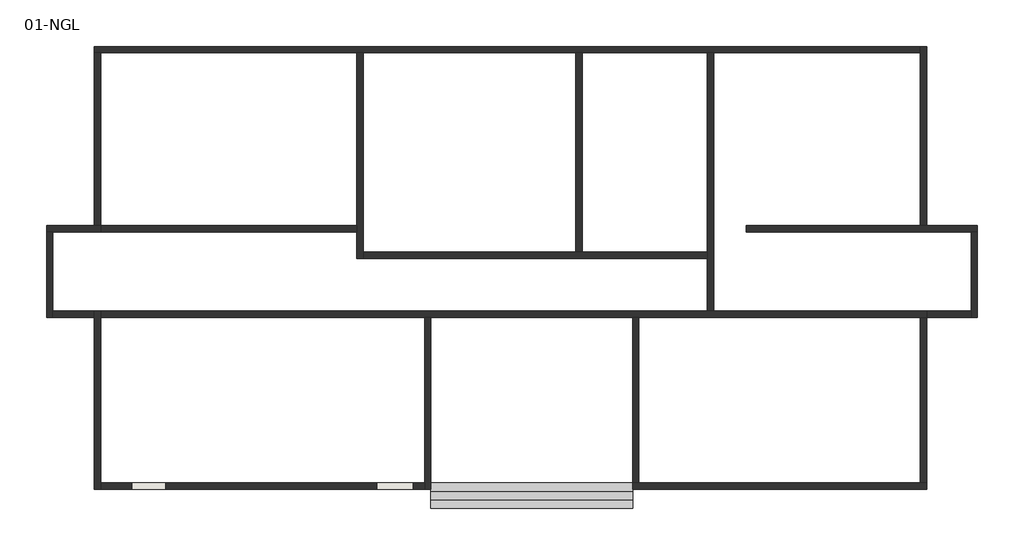
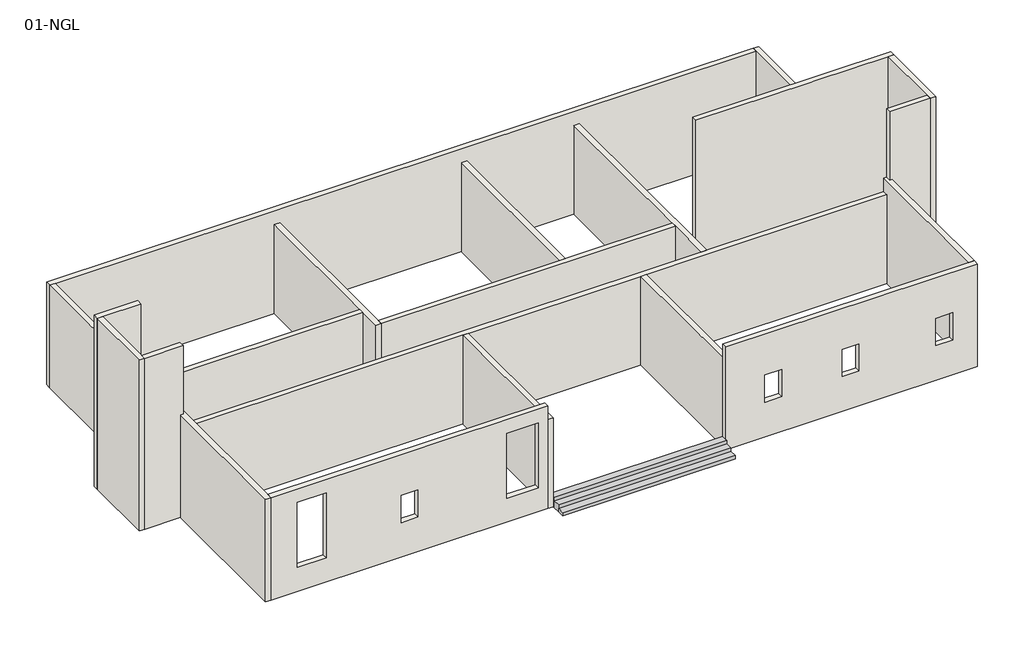
# One storey: 21 walls, 1 stair flight.
"""IFC4 building model written with IfcOpenShell, lengths in millimetres."""

from ifc_helpers import new_model, si_unit, frame, origin, origin_with_axes, place, context, project, spatial, polyline, outline, extrude, faceted_brep, element, save

model = new_model("IFC4")

# Units and contexts
model_context = context("Model", 3, world=origin())
ifc_project = project(units=[si_unit("LENGTHUNIT", "METRE", prefix="MILLI")], contexts=[model_context])

# Site, building, storey
site = spatial("IfcSite", under=ifc_project)
building = spatial("IfcBuilding", under=site)
storey = spatial("IfcBuildingStorey", under=building, Name="01-NGL", Elevation=0.0)

# Stair flight
placement = place(None, origin())
element("IfcStairFlight", 1, ObjectType="steps", at=placement, inside=storey, context=model_context, shape_type="Brep", body=[
    faceted_brep([(2218.5830368, -13353.0592374, 150.0), (2218.5830368, -13653.0592374, 150.0), (9368.5830368, -13653.0592374, 150.0), (9368.5830368, -13353.0592374, 150.0), (2218.5830368, -13353.0592374, 0.0), (2218.5830368, -13653.0592374, 0.0), (9368.5830368, -13653.0592374, 0.0), (9368.5830368, -13353.0592374, 0.0), (2218.5830368, -13053.0592374, 300.0), (2218.5830368, -13353.0592374, 300.0), (9368.5830368, -13353.0592374, 300.0), (9368.5830368, -13053.0592374, 300.0), (2218.5830368, -13053.0592374, 0.0), (9368.5830368, -13053.0592374, 0.0), (2218.5830368, -12753.0592374, 450.0), (2218.5830368, -13053.0592374, 450.0), (9368.5830368, -13053.0592374, 450.0), (9368.5830368, -12753.0592374, 450.0), (2218.5830368, -12753.0592374, 0.0), (9368.5830368, -12753.0592374, 0.0)], [[[0, 1, 2, 3]], [[1, 0, 4, 5]], [[2, 1, 5, 6]], [[3, 2, 6, 7]], [[8, 9, 10, 11]], [[4, 0, 9, 8, 12]], [[0, 3, 10, 9]], [[3, 7, 13, 11, 10]], [[14, 15, 16, 17]], [[12, 8, 15, 14, 18]], [[8, 11, 16, 15]], [[11, 13, 19, 17, 16]], [[14, 17, 19, 18]], [[5, 4, 12, 18, 19, 13, 7, 6]]]),
])

# Walls
element("IfcWall", 2, ObjectType="01-225 WALL", at=placement, inside=storey, context=model_context, shape_type="Brep", body=[
    faceted_brep([(-9718.9169632, 2521.9407626, 0.0), (-9493.9169632, 2521.9407626, 0.0), (-406.4169632, 2521.9407626, 0.0), (-181.4169632, 2521.9407626, 0.0), (7356.0830368, 2521.9407626, 0.0), (7581.0830368, 2521.9407626, 0.0), (12021.0830368, 2521.9407626, 0.0), (12246.0830368, 2521.9407626, 0.0), (19581.0830368, 2521.9407626, 0.0), (19581.0830368, 2521.9407626, 4500.0), (-9493.9169632, 2521.9407626, 4500.0), (-9718.9169632, 2521.9407626, 4500.0), (-9718.9169632, 2746.9407626, 0.0), (-9718.9169632, 2746.9407626, 4500.0), (19581.0830368, 2746.9407626, 4500.0), (19581.0830368, 2746.9407626, 0.0)], [[[0, 1, 2, 3, 4, 5, 6, 7, 8, 9, 10, 11]], [[12, 13, 14, 15]], [[8, 7, 6, 5, 4, 3, 2, 1, 0, 12, 15]], [[11, 10, 9, 14, 13]], [[0, 11, 13, 12]], [[9, 8, 15, 14]]]),
])
element("IfcWall", 3, ObjectType="01-225 WALL", at=placement, inside=storey, context=model_context, shape_type="Brep", body=[
    faceted_brep([(-9493.9169632, -12978.0592374, 0.0), (-9493.9169632, -12753.0592374, 0.0), (-9493.9169632, -6865.5592374, 0.0), (-9493.9169632, -6640.5592374, 0.0), (-9493.9169632, -6640.5592374, 3900.0), (-9493.9169632, -6640.5592374, 4500.0), (-9493.9169632, -6865.5592374, 4500.0), (-9493.9169632, -12753.0592374, 4500.0), (-9493.9169632, -12978.0592374, 4500.0), (-9718.9169632, -12978.0592374, 0.0), (-9718.9169632, -12978.0592374, 4500.0), (-9718.9169632, -6865.5592374, 4500.0), (-9718.9169632, -6640.5592374, 4500.0), (-9718.9169632, -6640.5592374, 0.0), (-9718.9169632, -6865.5592374, 0.0), (-9606.4169632, -6640.5592374, 4500.0)], [[[0, 1, 2, 3, 4, 5, 6, 7, 8]], [[9, 10, 11, 12, 13, 14]], [[3, 2, 1, 0, 9, 14, 13]], [[8, 7, 6, 5, 15, 12, 11, 10]], [[0, 8, 10, 9]], [[3, 13, 12, 15, 5, 4]]]),
])
element("IfcWall", 4, ObjectType="01-225 WALL", at=placement, inside=storey, context=model_context, shape_type="Brep", body=[
    faceted_brep([(19806.0830368, -12753.0592374, 0.0), (19581.0830368, -12753.0592374, 0.0), (9593.5830368, -12753.0592374, 0.0), (9368.5830368, -12753.0592374, 0.0), (9368.5830368, -12753.0592374, 3900.0), (9368.5830368, -12753.0592374, 4500.0), (19581.0830368, -12753.0592374, 4500.0), (19806.0830368, -12753.0592374, 4500.0), (11693.5830368, -12753.0592374, 2714.4), (10993.5830368, -12753.0592374, 2714.4), (10993.5830368, -12753.0592374, 1514.4), (11693.5830368, -12753.0592374, 1514.4), (14193.5830368, -12753.0592374, 2714.4), (14193.5830368, -12753.0592374, 1514.4), (14893.5830368, -12753.0592374, 1514.4), (14893.5830368, -12753.0592374, 2714.4), (18081.0830368, -12753.0592374, 2714.4), (18081.0830368, -12753.0592374, 1514.4), (18781.0830368, -12753.0592374, 1514.4), (18781.0830368, -12753.0592374, 2714.4), (19806.0830368, -12978.0592374, 0.0), (19806.0830368, -12978.0592374, 4500.0), (9368.5830368, -12978.0592374, 4500.0), (9368.5830368, -12978.0592374, 0.0), (11693.5830368, -12978.0592374, 2714.4), (11693.5830368, -12978.0592374, 1514.4), (10993.5830368, -12978.0592374, 1514.4), (10993.5830368, -12978.0592374, 2714.4), (14193.5830368, -12978.0592374, 2714.4), (14893.5830368, -12978.0592374, 2714.4), (14893.5830368, -12978.0592374, 1514.4), (14193.5830368, -12978.0592374, 1514.4), (18081.0830368, -12978.0592374, 2714.4), (18781.0830368, -12978.0592374, 2714.4), (18781.0830368, -12978.0592374, 1514.4), (18081.0830368, -12978.0592374, 1514.4)], [[[0, 1, 2, 3, 4, 5, 6, 7], [8, 9, 10, 11], [12, 13, 14, 15], [16, 17, 18, 19]], [[20, 21, 22, 23], [24, 25, 26, 27], [28, 29, 30, 31], [32, 33, 34, 35]], [[3, 2, 1, 0, 20, 23]], [[7, 6, 5, 22, 21]], [[0, 7, 21, 20]], [[5, 4, 3, 23, 22]], [[25, 24, 8, 11]], [[26, 25, 11, 10]], [[27, 26, 10, 9]], [[24, 27, 9, 8]], [[13, 12, 28, 31]], [[14, 13, 31, 30]], [[15, 14, 30, 29]], [[12, 15, 29, 28]], [[17, 16, 32, 35]], [[18, 17, 35, 34]], [[19, 18, 34, 33]], [[16, 19, 33, 32]]]),
])
element("IfcWall", 5, ObjectType="01-225 WALL", at=placement, inside=storey, context=model_context, shape_type="Brep", body=[
    faceted_brep([(19581.0830368, 2746.9407626, 0.0), (19581.0830368, 2521.9407626, 0.0), (19581.0830368, -3615.5592374, 0.0), (19581.0830368, -3615.5592374, 4500.0), (19581.0830368, 2521.9407626, 4500.0), (19581.0830368, 2746.9407626, 4500.0), (19806.0830368, 2746.9407626, 0.0), (19806.0830368, 2746.9407626, 4500.0), (19806.0830368, -3615.5592374, 4500.0), (19806.0830368, -3615.5592374, 0.0)], [[[0, 1, 2, 3, 4, 5]], [[6, 7, 8, 9]], [[2, 1, 0, 6, 9]], [[5, 4, 3, 8, 7]], [[0, 5, 7, 6]], [[3, 2, 9, 8]]]),
])
element("IfcWall", 6, ObjectType="01-225 WALL", at=placement, inside=storey, context=model_context, shape_type="Brep", body=[
    faceted_brep([(-9493.9169632, -6865.5592374, 0.0), (1993.5830368, -6865.5592374, 0.0), (2218.5830368, -6865.5592374, 0.0), (9368.5830368, -6865.5592374, 0.0), (9593.5830368, -6865.5592374, 0.0), (19581.0830368, -6865.5592374, 0.0), (19806.0830368, -6865.5592374, 0.0), (19806.0830368, -6865.5592374, 3900.0), (19581.0830368, -6865.5592374, 3900.0), (9593.5830368, -6865.5592374, 3900.0), (9368.5830368, -6865.5592374, 3900.0), (2218.5830368, -6865.5592374, 3900.0), (1993.5830368, -6865.5592374, 3900.0), (-9493.9169632, -6865.5592374, 3900.0), (-9493.9169632, -6640.5592374, 0.0), (-9493.9169632, -6640.5592374, 3900.0), (1993.5830368, -6640.5592374, 3900.0), (9593.5830368, -6640.5592374, 3900.0), (12021.0830368, -6640.5592374, 3900.0), (12246.0830368, -6640.5592374, 3900.0), (19581.0830368, -6640.5592374, 3900.0), (19806.0830368, -6640.5592374, 3900.0), (19806.0830368, -6640.5592374, 0.0), (12246.0830368, -6640.5592374, 0.0), (12021.0830368, -6640.5592374, 0.0)], [[[0, 1, 2, 3, 4, 5, 6, 7, 8, 9, 10, 11, 12, 13]], [[14, 15, 16, 17, 18, 19, 20, 21, 22, 23, 24]], [[6, 5, 4, 3, 2, 1, 0, 14, 24, 23, 22]], [[13, 12, 11, 10, 9, 8, 7, 21, 20, 19, 18, 17, 16, 15]], [[0, 13, 15, 14]], [[7, 6, 22, 21]]]),
])
element("IfcWall", 7, ObjectType="01-225 WALL", at=placement, inside=storey, context=model_context, shape_type="Brep", body=[
    faceted_brep([(2218.5830368, -12978.0592374, 0.0), (2218.5830368, -6865.5592374, 0.0), (2218.5830368, -6865.5592374, 3900.0), (2218.5830368, -12978.0592374, 3900.0), (1993.5830368, -12978.0592374, 0.0), (1993.5830368, -12978.0592374, 3900.0), (1993.5830368, -6865.5592374, 3900.0), (1993.5830368, -6865.5592374, 0.0), (1993.5830368, -12753.0592374, 0.0)], [[[0, 1, 2, 3]], [[4, 5, 6, 7, 8]], [[1, 0, 4, 8, 7]], [[3, 2, 6, 5]], [[2, 1, 7, 6]], [[0, 3, 5, 4]]]),
])
element("IfcWall", 8, ObjectType="01-225 WALL", at=placement, inside=storey, context=model_context, shape_type="SweptSolid", body=[
    extrude(outline(polyline([(9368.5830368, -12753.0592374), (9368.5830368, -6865.5592374), (9593.5830368, -6865.5592374), (9593.5830368, -12753.0592374), (9368.5830368, -12753.0592374)])), origin_with_axes(), (0.0, 0.0, 1.0), 3900.0),
])
element("IfcWall", 9, ObjectType="01-225 WALL", at=placement, inside=storey, context=model_context, shape_type="Brep", body=[
    faceted_brep([(12021.0830368, 2521.9407626, 0.0), (12021.0830368, -4553.0592374, 0.0), (12021.0830368, -4778.0592374, 0.0), (12021.0830368, -6640.5592374, 0.0), (12021.0830368, -6640.5592374, 3900.0), (12021.0830368, -4778.0592374, 3900.0), (12021.0830368, -4553.0592374, 3900.0), (12021.0830368, 2521.9407626, 3900.0), (12246.0830368, 2521.9407626, 0.0), (12246.0830368, 2521.9407626, 3900.0), (12246.0830368, -6640.5592374, 3900.0), (12246.0830368, -6640.5592374, 0.0)], [[[0, 1, 2, 3, 4, 5, 6, 7]], [[8, 9, 10, 11]], [[3, 2, 1, 0, 8, 11]], [[7, 6, 5, 4, 10, 9]], [[0, 7, 9, 8]], [[4, 3, 11, 10]]]),
])
element("IfcWall", 10, ObjectType="01-225 WALL", at=placement, inside=storey, context=model_context, shape_type="Brep", body=[
    faceted_brep([(-406.4169632, 2521.9407626, 0.0), (-406.4169632, -3615.5592374, 0.0), (-406.4169632, -3840.5592374, 0.0), (-406.4169632, -4778.0592374, 0.0), (-406.4169632, -4778.0592374, 3900.0), (-406.4169632, -3840.5592374, 3900.0), (-406.4169632, -3615.5592374, 3900.0), (-406.4169632, 2521.9407626, 3900.0), (-181.4169632, 2521.9407626, 0.0), (-181.4169632, 2521.9407626, 3900.0), (-181.4169632, -4553.0592374, 3900.0), (-181.4169632, -4778.0592374, 3900.0), (-181.4169632, -4778.0592374, 0.0), (-181.4169632, -4553.0592374, 0.0)], [[[0, 1, 2, 3, 4, 5, 6, 7]], [[8, 9, 10, 11, 12, 13]], [[3, 2, 1, 0, 8, 13, 12]], [[7, 6, 5, 4, 11, 10, 9]], [[0, 7, 9, 8]], [[4, 3, 12, 11]]]),
])
element("IfcWall", 11, ObjectType="01-225 WALL", at=placement, inside=storey, context=model_context, shape_type="Brep", body=[
    faceted_brep([(-181.4169632, -4778.0592374, 0.0), (12021.0830368, -4778.0592374, 0.0), (12021.0830368, -4778.0592374, 3900.0), (-181.4169632, -4778.0592374, 3900.0), (-181.4169632, -4553.0592374, 0.0), (-181.4169632, -4553.0592374, 3900.0), (7356.0830368, -4553.0592374, 3900.0), (7581.0830368, -4553.0592374, 3900.0), (12021.0830368, -4553.0592374, 3900.0), (12021.0830368, -4553.0592374, 0.0), (7581.0830368, -4553.0592374, 0.0), (7356.0830368, -4553.0592374, 0.0)], [[[0, 1, 2, 3]], [[4, 5, 6, 7, 8, 9, 10, 11]], [[1, 0, 4, 11, 10, 9]], [[3, 2, 8, 7, 6, 5]], [[2, 1, 9, 8]], [[0, 3, 5, 4]]]),
])
element("IfcWall", 12, ObjectType="01-225 WALL", at=placement, inside=storey, context=model_context, shape_type="SweptSolid", body=[
    extrude(outline(polyline([(7356.0830368, -4553.0592374), (7356.0830368, 2521.9407626), (7581.0830368, 2521.9407626), (7581.0830368, -4553.0592374), (7356.0830368, -4553.0592374)])), origin_with_axes(), (0.0, 0.0, 1.0), 3900.0),
])
element("IfcWall", 13, ObjectType="01-225 WALL", at=placement, inside=storey, context=model_context, shape_type="SweptSolid", body=[
    extrude(outline(polyline([(-9493.9169632, -3615.5592374), (-406.4169632, -3615.5592374), (-406.4169632, -3840.5592374), (-9493.9169632, -3840.5592374), (-9493.9169632, -3615.5592374)])), origin_with_axes(), (0.0, 0.0, 1.0), 3900.0),
])
element("IfcWall", 14, ObjectType="01-225 WALL", at=placement, inside=storey, context=model_context, shape_type="Brep", body=[
    faceted_brep([(-9493.9169632, -3615.5592374, 4500.0), (-9493.9169632, -3615.5592374, 3900.0), (-9493.9169632, -3615.5592374, 0.0), (-9718.9169632, -3615.5592374, 0.0), (-11418.9169632, -3615.5592374, 0.0), (-11418.9169632, -3615.5592374, 7500.0), (-9606.4169632, -3615.5592374, 7500.0), (-9606.4169632, -3615.5592374, 4500.0), (-9493.9169632, -3840.5592374, 0.0), (-9493.9169632, -3840.5592374, 3900.0), (-9493.9169632, -3840.5592374, 4500.0), (-9606.4169632, -3840.5592374, 4500.0), (-9606.4169632, -3840.5592374, 7500.0), (-11193.9169632, -3840.5592374, 7500.0), (-11418.9169632, -3840.5592374, 7500.0), (-11418.9169632, -3840.5592374, 0.0), (-11193.9169632, -3840.5592374, 0.0)], [[[0, 1, 2, 3, 4, 5, 6, 7]], [[8, 9, 10, 11, 12, 13, 14, 15, 16]], [[4, 3, 2, 8, 16, 15]], [[6, 5, 14, 13, 12]], [[5, 4, 15, 14]], [[7, 6, 12, 11]], [[7, 11, 10, 0]], [[0, 10, 9, 8, 2, 1]]]),
])
element("IfcWall", 15, ObjectType="01-225 WALL", at=placement, inside=storey, context=model_context, shape_type="Brep", body=[
    faceted_brep([(-11418.9169632, -3840.5592374, 0.0), (-11418.9169632, -6865.5592374, 0.0), (-11418.9169632, -6865.5592374, 7500.0), (-11418.9169632, -3840.5592374, 7500.0), (-11193.9169632, -3840.5592374, 0.0), (-11193.9169632, -3840.5592374, 7500.0), (-11193.9169632, -6640.5592374, 7500.0), (-11193.9169632, -6865.5592374, 7500.0), (-11193.9169632, -6865.5592374, 0.0), (-11193.9169632, -6640.5592374, 0.0)], [[[0, 1, 2, 3]], [[4, 5, 6, 7, 8, 9]], [[1, 0, 4, 9, 8]], [[3, 2, 7, 6, 5]], [[0, 3, 5, 4]], [[2, 1, 8, 7]]]),
])
element("IfcWall", 16, ObjectType="01-225 WALL", at=placement, inside=storey, context=model_context, shape_type="SweptSolid", body=[
    extrude(outline(polyline([(0.0, -11193.9169632), (0.0, -9718.9169632), (4500.0, -9718.9169632), (4500.0, -9606.4169632), (7500.0, -9606.4169632), (7500.0, -11193.9169632), (0.0, -11193.9169632)])), frame((0.0, -6865.5592374, 0.0), z_axis=(0.0, 1.0, 0.0), x_axis=(0.0, 0.0, 1.0)), (0.0, 0.0, 1.0), 225.0),
])
element("IfcWall", 17, ObjectType="01-225 WALL", at=placement, inside=storey, context=model_context, shape_type="Brep", body=[
    faceted_brep([(13406.0415807, -3840.5592374, 0.0), (21381.0830368, -3840.5592374, 0.0), (21606.0830368, -3840.5592374, 0.0), (21606.0830368, -3840.5592374, 7500.0), (21381.0830368, -3840.5592374, 7500.0), (18353.5830368, -3840.5592374, 7500.0), (18128.5830368, -3840.5592374, 7500.0), (13406.0415807, -3840.5592374, 7500.0), (13406.0415807, -3840.5592374, 3900.0), (13406.0415807, -3615.5592374, 0.0), (13406.0415807, -3615.5592374, 3900.0), (13406.0415807, -3615.5592374, 7500.0), (21606.0830368, -3615.5592374, 7500.0), (21606.0830368, -3615.5592374, 0.0), (19806.0830368, -3615.5592374, 0.0), (19581.0830368, -3615.5592374, 0.0)], [[[0, 1, 2, 3, 4, 5, 6, 7, 8]], [[9, 10, 11, 12, 13, 14, 15]], [[2, 1, 0, 9, 15, 14, 13]], [[7, 6, 5, 4, 3, 12, 11]], [[0, 8, 7, 11, 10, 9]], [[3, 2, 13, 12]]]),
])
element("IfcWall", 18, ObjectType="01-225 WALL", at=placement, inside=storey, context=model_context, shape_type="Brep", body=[
    faceted_brep([(21381.0830368, -3840.5592374, 0.0), (21381.0830368, -6640.5592374, 0.0), (21381.0830368, -6865.5592374, 0.0), (21381.0830368, -6865.5592374, 7500.0), (21381.0830368, -6640.5592374, 7500.0), (21381.0830368, -3840.5592374, 7500.0), (21606.0830368, -3840.5592374, 0.0), (21606.0830368, -3840.5592374, 7500.0), (21606.0830368, -6865.5592374, 7500.0), (21606.0830368, -6865.5592374, 0.0)], [[[0, 1, 2, 3, 4, 5]], [[6, 7, 8, 9]], [[2, 1, 0, 6, 9]], [[5, 4, 3, 8, 7]], [[0, 5, 7, 6]], [[3, 2, 9, 8]]]),
])
element("IfcWall", 19, ObjectType="01-225 WALL", at=placement, inside=storey, context=model_context, shape_type="Brep", body=[
    faceted_brep([(21381.0830368, -6640.5592374, 0.0), (19806.0830368, -6640.5592374, 0.0), (19806.0830368, -6640.5592374, 3900.0), (19806.0830368, -6640.5592374, 4500.0), (19693.5830368, -6640.5592374, 4500.0), (19693.5830368, -6640.5592374, 7500.0), (21381.0830368, -6640.5592374, 7500.0), (21381.0830368, -6865.5592374, 0.0), (21381.0830368, -6865.5592374, 7500.0), (19693.5830368, -6865.5592374, 7500.0), (19693.5830368, -6865.5592374, 4500.0), (19806.0830368, -6865.5592374, 4500.0), (19806.0830368, -6865.5592374, 3900.0), (19806.0830368, -6865.5592374, 0.0)], [[[0, 1, 2, 3, 4, 5, 6]], [[7, 8, 9, 10, 11, 12, 13]], [[1, 0, 7, 13]], [[6, 5, 9, 8]], [[0, 6, 8, 7]], [[5, 4, 10, 9]], [[10, 4, 3, 11]], [[1, 13, 12, 11, 3, 2]]]),
])
element("IfcWall", 20, ObjectType="01-225 WALL", at=placement, inside=storey, context=model_context, shape_type="Brep", body=[
    faceted_brep([(-9493.9169632, -3615.5592374, 4500.0), (-9493.9169632, -3615.5592374, 0.0), (-9493.9169632, 2521.9407626, 0.0), (-9493.9169632, 2521.9407626, 4500.0), (-9718.9169632, -3615.5592374, 0.0), (-9718.9169632, -3615.5592374, 4500.0), (-9718.9169632, 2521.9407626, 4500.0), (-9718.9169632, 2521.9407626, 0.0), (-9606.4169632, -3615.5592374, 4500.0)], [[[0, 1, 2, 3]], [[4, 5, 6, 7]], [[2, 1, 4, 7]], [[0, 3, 6, 5, 8]], [[3, 2, 7, 6]], [[0, 8, 5, 4, 1]]]),
])
element("IfcWall", 21, ObjectType="01-225 WALL", at=placement, inside=storey, context=model_context, shape_type="Brep", body=[
    faceted_brep([(19581.0830368, -6865.5592374, 0.0), (19581.0830368, -12753.0592374, 0.0), (19581.0830368, -12753.0592374, 4500.0), (19581.0830368, -6865.5592374, 4500.0), (19581.0830368, -6640.5592374, 4500.0), (19581.0830368, -6640.5592374, 3900.0), (19581.0830368, -6865.5592374, 3900.0), (19806.0830368, -6865.5592374, 0.0), (19806.0830368, -6865.5592374, 3900.0), (19806.0830368, -6640.5592374, 3900.0), (19806.0830368, -6640.5592374, 4500.0), (19806.0830368, -6865.5592374, 4500.0), (19806.0830368, -12753.0592374, 4500.0), (19806.0830368, -12753.0592374, 0.0), (19693.5830368, -6640.5592374, 4500.0)], [[[0, 1, 2, 3, 4, 5, 6]], [[7, 8, 9, 10, 11, 12, 13]], [[1, 0, 7, 13]], [[4, 3, 2, 12, 11, 10, 14]], [[2, 1, 13, 12]], [[5, 9, 8, 6]], [[0, 6, 8, 7]], [[5, 4, 14, 10, 9]]]),
])
element("IfcWall", 22, ObjectType="01-225 WALL", at=placement, inside=storey, context=model_context, shape_type="Brep", body=[
    faceted_brep([(1993.5830368, -12753.0592374, 0.0), (-9493.9169632, -12753.0592374, 0.0), (-9493.9169632, -12753.0592374, 4500.0), (1993.5830368, -12753.0592374, 4500.0), (-8393.9169632, -12753.0592374, 3900.0), (-8393.9169632, -12753.0592374, 1050.0), (-7193.9169632, -12753.0592374, 1050.0), (-7193.9169632, -12753.0592374, 3900.0), (1593.5830368, -12753.0592374, 1050.0), (1593.5830368, -12753.0592374, 3900.0), (293.5830368, -12753.0592374, 3900.0), (293.5830368, -12753.0592374, 1050.0), (-4093.9169632, -12753.0592374, 2714.4), (-4093.9169632, -12753.0592374, 1514.4), (-3393.9169632, -12753.0592374, 1514.4), (-3393.9169632, -12753.0592374, 2714.4), (-9493.9169632, -12978.0592374, 0.0), (1993.5830368, -12978.0592374, 0.0), (1993.5830368, -12978.0592374, 3900.0), (1993.5830368, -12978.0592374, 4500.0), (-9493.9169632, -12978.0592374, 4500.0), (-8393.9169632, -12978.0592374, 1050.0), (-8393.9169632, -12978.0592374, 3900.0), (-7193.9169632, -12978.0592374, 3900.0), (-7193.9169632, -12978.0592374, 1050.0), (1593.5830368, -12978.0592374, 3900.0), (1593.5830368, -12978.0592374, 1050.0), (293.5830368, -12978.0592374, 1050.0), (293.5830368, -12978.0592374, 3900.0), (-4093.9169632, -12978.0592374, 2714.4), (-3393.9169632, -12978.0592374, 2714.4), (-3393.9169632, -12978.0592374, 1514.4), (-4093.9169632, -12978.0592374, 1514.4)], [[[0, 1, 2, 3], [4, 5, 6, 7], [8, 9, 10, 11], [12, 13, 14, 15]], [[16, 17, 18, 19, 20], [21, 22, 23, 24], [25, 26, 27, 28], [29, 30, 31, 32]], [[1, 0, 17, 16]], [[3, 2, 20, 19]], [[2, 1, 16, 20]], [[0, 3, 19, 18, 17]], [[21, 5, 4, 22]], [[22, 4, 7, 23]], [[23, 7, 6, 24]], [[5, 21, 24, 6]], [[8, 26, 25, 9]], [[9, 25, 28, 10]], [[10, 28, 27, 11]], [[26, 8, 11, 27]], [[13, 12, 29, 32]], [[14, 13, 32, 31]], [[15, 14, 31, 30]], [[12, 15, 30, 29]]]),
])

save(model, "model.ifc")

# Revit data of these elements
# Type "01-225 WALL"
#   Description = "Generic Wall (Material By Category), 200mm thick"
#   Assembly Code = "B2010"
#   Type Mark = "G06"
#   Layers, outside or top first: 225 mm "01-WHITE WALL" (function 1)
# Element 1 (IfcStairFlight, "steps")
#   Phase Created = New Construction
# Elements 2, 3, 4, 5, 20, 21, 22 (IfcWall, "01-225 WALL")
#   Top Offset = 0 mm
#   Base Offset = 0 mm
#   wall height = 4500 mm
#   Phase Created = New Construction
#   Base Constraint = 01-NGL
#   Top Constraint = 05-ROOF LEVEL
#   Materials on its faces: "01-WHITE WALL"
# Elements 6, 7, 8, 9, 10, 11, 12, 13 (IfcWall, "01-225 WALL")
#   Top Offset = 0 mm
#   Base Offset = 0 mm
#   wall height = 3900 mm
#   Phase Created = New Construction
#   Base Constraint = 01-NGL
#   Top Constraint = 04-CEILING
#   Materials on its faces: "01-WHITE WALL"
# Elements 14, 15, 16, 17, 18, 19 (IfcWall, "01-225 WALL")
#   Top Offset = 0 mm
#   Base Offset = 0 mm
#   wall height = 7500 mm
#   Phase Created = New Construction
#   Base Constraint = 01-NGL
#   Materials on its faces: "01-WHITE WALL"
# Materials
#   "01-WHITE WALL": class "Generic", colour RGB 244 244 244, transparency 0, Description = "Acoustic Ceiling Tile 24 x 48", Cost = 0
